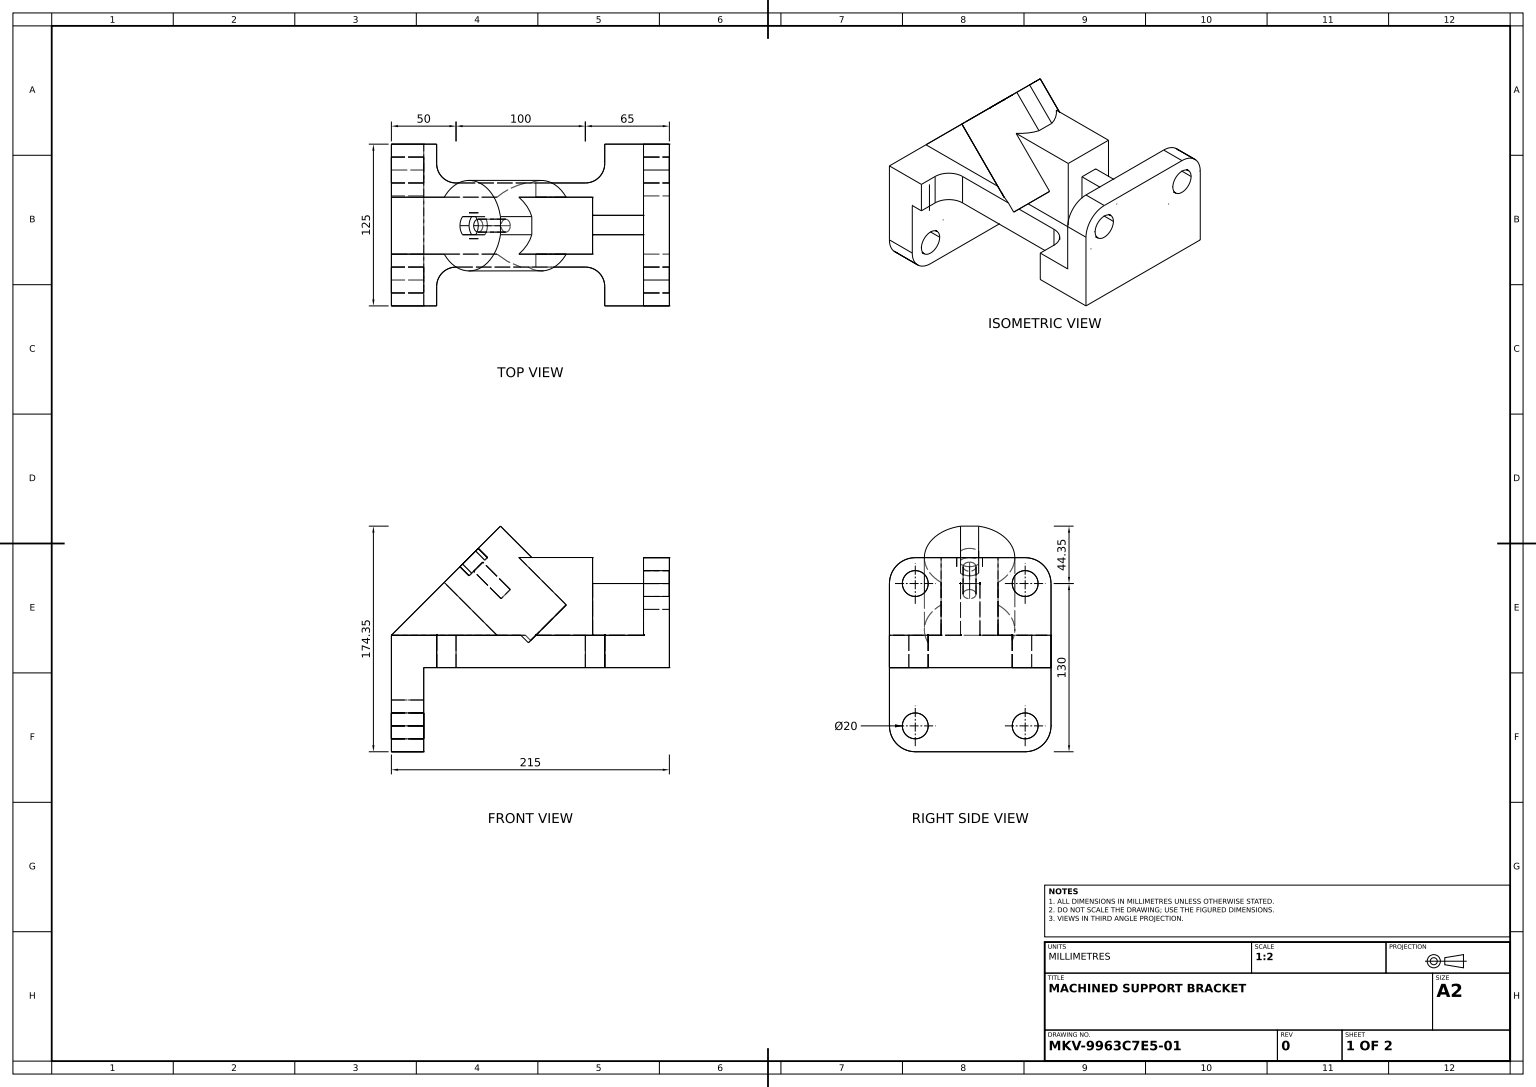
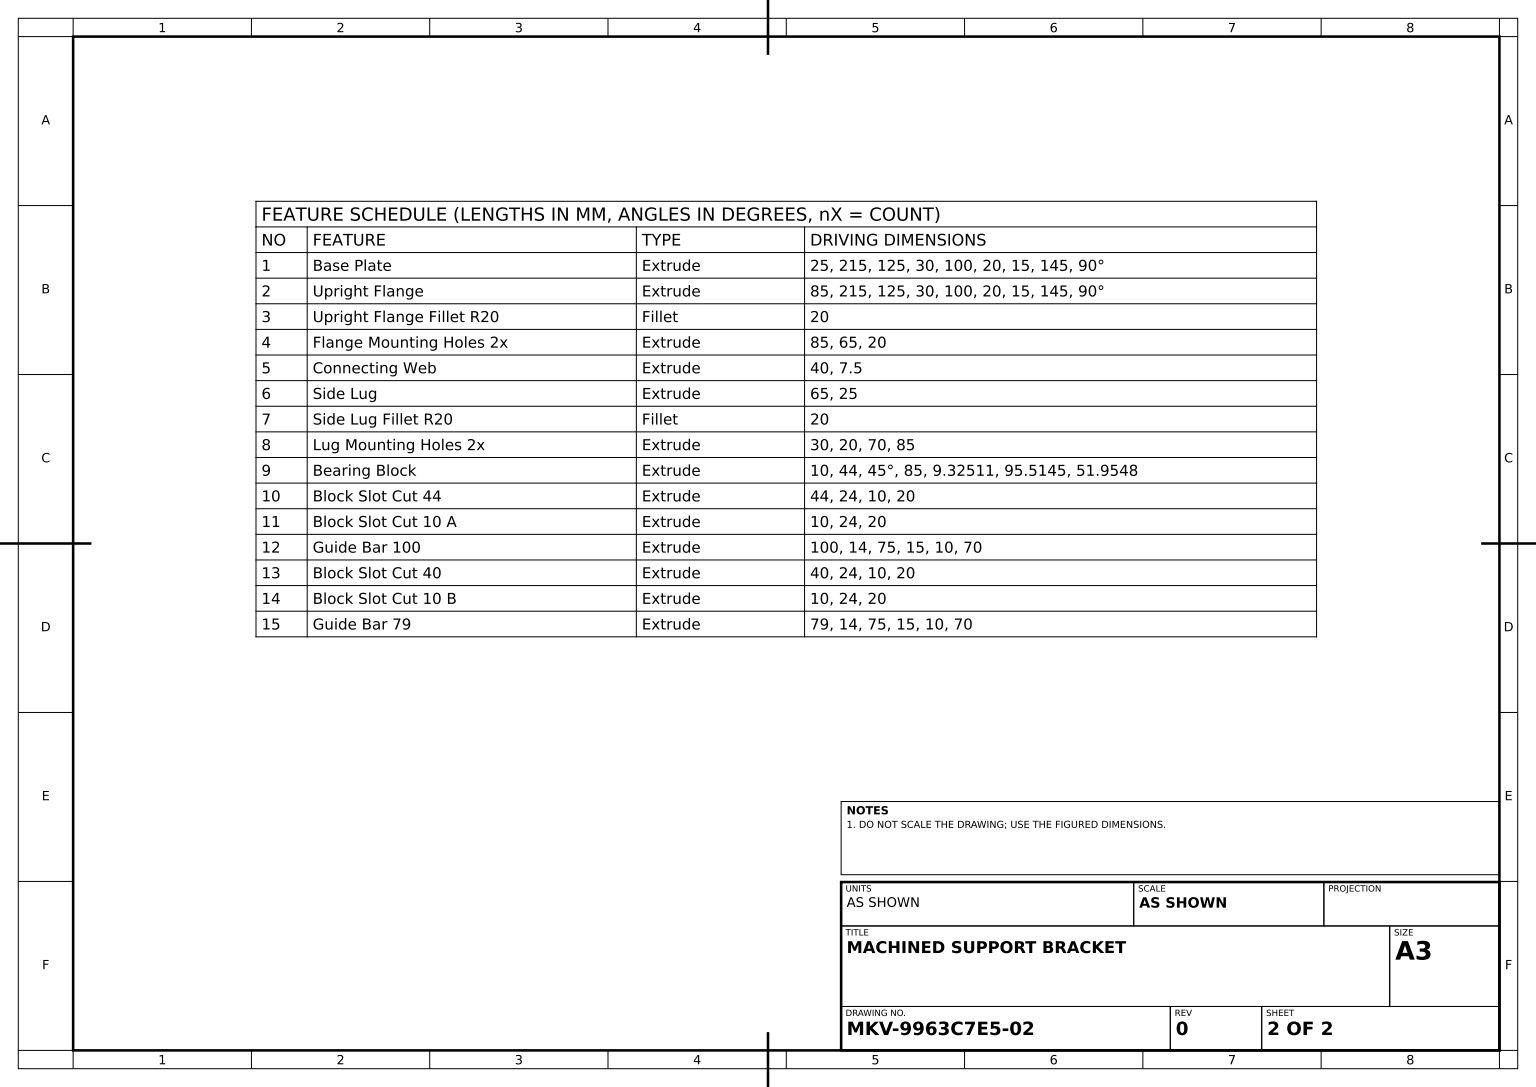
from build123d import *
from build123d.topology import SkipClean

# Parameters (mm, degrees)
BASE_PLATE_DEPTH               = 25
SKETCH1_3_W                    = 20
SKETCH1_3_H                    = 62.5
UPRIGHT_FLANGE_DEPTH           = 85
UPRIGHT_FLANGE_FILLET_R20_R    = 20
FLANGE_HOLES_SKETCH_R          = 10
FLANGE_MOUNTING_HOLES_2X_DEPTH = 85
CONNECTING_WEB_SKETCH_W        = 40
CONNECTING_WEB_SKETCH_H        = 15
CONNECTING_WEB_DEPTH           = 40
SIDE_LUG_SKETCH_W              = 25
SIDE_LUG_SKETCH_H              = 125
SIDE_LUG_DEPTH                 = 65
SIDE_LUG_FILLET_R20_R          = 20
LUG_HOLES_SKETCH_R             = 10
LUG_MOUNTING_HOLES_2X_DEPTH    = 30
BEARING_BLOCK_DEPTH            = 44
BLOCK_SLOT_SKETCH_R            = 5
BLOCK_SLOT_CUT_44_DEPTH        = 44
SKETCH12_4_R                   = 10
SKETCH12_4_R_2                 = 5
BLOCK_SLOT_CUT_10_A_DEPTH      = 10
GUIDE_BAR_SKETCH_W             = 14
GUIDE_BAR_SKETCH_H             = 44.292856399
GUIDE_BAR_100_DEPTH            = 100
SKETCH12_5_R                   = 5
BLOCK_SLOT_CUT_40_DEPTH        = 40
SKETCH12_6_R                   = 10
SKETCH12_6_R_2                 = 5
BLOCK_SLOT_CUT_10_B_DEPTH      = 10
GUIDE_BAR_79_DEPTH             = 79


with BuildPart() as part:
    # Base Profile Sketch → Base Plate (new body)
    with BuildSketch(Plane(origin=(0, 0, 0), x_dir=(1, 0, 0), z_dir=(0, 1, 0))):
        with BuildLine():
            Line((0, 62.5), (0, 0))
            Line((0, 0), (35, 0))
            Line((35, 0), (35, 15))
            ThreePointArc((35, 15), (39.393398282, 25.606601718), (50, 30))
            Line((50, 30), (150, 30))
            ThreePointArc((150, 30), (160.606601718, 25.606601718), (165, 15))
            Line((165, 15), (165, 0))
            Line((165, 0), (195, 0))
            Line((195, 0), (195, 62.5))
            Line((195, 62.5), (0, 62.5))
        make_face()
        with BuildLine():
            Line((0, 125), (0, 62.5))
            Line((0, 62.5), (195, 62.5))
            Line((195, 62.5), (195, 125))
            Line((195, 125), (165, 125))
            Line((165, 125), (165, 110))
            ThreePointArc((165, 110), (160.606601718, 99.393398282), (150, 95))
            Line((150, 95), (50, 95))
            ThreePointArc((50, 95), (39.393398282, 99.393398282), (35, 110))
            Line((35, 110), (35, 125))
            Line((35, 125), (0, 125))
        make_face()
    extrude(amount=BASE_PLATE_DEPTH)

    # Sketch1_3 → Upright Flange (add)
    with BuildSketch(Plane(origin=(0, 0, 0), x_dir=(1, 0, 0), z_dir=(0, 1, 0))):
        with Locations((205, 31.25)):
            Rectangle(SKETCH1_3_W, SKETCH1_3_H)
        with Locations((205, 93.75)):
            Rectangle(SKETCH1_3_W, SKETCH1_3_H)
    extrude(amount=UPRIGHT_FLANGE_DEPTH)

    # Upright Flange Fillet R20
    upright_flange_fillet_r20_edges = [part.edges().sort_by_distance(p)[0] for p in [
        (205, 85, 0),
        (205, 85, -125),
    ]]
    fillet(upright_flange_fillet_r20_edges, radius=UPRIGHT_FLANGE_FILLET_R20_R)

    # Flange Holes Sketch → Flange Mounting Holes 2x (cut)
    with BuildSketch(Plane(origin=(215, 0, 0), x_dir=(0, 0, -1), z_dir=(1, 0, 0))):
        with Locations((20, 65)):
            Circle(FLANGE_HOLES_SKETCH_R)
        with Locations((105, 65)):
            Circle(FLANGE_HOLES_SKETCH_R)
    extrude(amount=-FLANGE_MOUNTING_HOLES_2X_DEPTH, mode=Mode.SUBTRACT)

    # Connecting Web Sketch → Connecting Web (add)
    with BuildSketch(Plane(origin=(0, 25, 0), x_dir=(1, 0, 0), z_dir=(0, 1, 0))):
        with Locations((175, 62.5)):
            Rectangle(CONNECTING_WEB_SKETCH_W, CONNECTING_WEB_SKETCH_H)
    extrude(amount=CONNECTING_WEB_DEPTH)

    # Side Lug Sketch → Side Lug (add)
    with BuildSketch(Plane(origin=(0, 0, 0), x_dir=(-1, 0, 0), z_dir=(0, -1, 0))):
        with Locations((-12.5, 62.5)):
            Rectangle(SIDE_LUG_SKETCH_W, SIDE_LUG_SKETCH_H)
    extrude(amount=SIDE_LUG_DEPTH)

    # Side Lug Fillet R20
    side_lug_fillet_r20_edges = [part.edges().sort_by_distance(p)[0] for p in [
        (12.5, -65, 0),
        (12.5, -65, -125),
    ]]
    fillet(side_lug_fillet_r20_edges, radius=SIDE_LUG_FILLET_R20_R)

    # Lug Holes Sketch → Lug Mounting Holes 2x (cut)
    with BuildSketch(Plane.ZY):
        with Locations((-105, -45)):
            Circle(LUG_HOLES_SKETCH_R)
        with Locations((-20, -45)):
            Circle(LUG_HOLES_SKETCH_R)
    extrude(amount=-LUG_MOUNTING_HOLES_2X_DEPTH, mode=Mode.SUBTRACT)

    # Bearing Block Profile Sketch → Bearing Block (add)
    with BuildSketch(Plane.XY.offset(-40)):
        Polygon((0, 25), (60.104076401, 85.104076401), (146.293439814, 85.104076401), (155.618552468, 85.104076401), (155.618552468, 76.954753414), (155.618552468, 25), align=None)
    extrude(amount=-BEARING_BLOCK_DEPTH)

    # Block Slot Sketch → Block Slot Cut 44 (cut)
    with BuildSketch(Plane(origin=(-12.5, 12.5, 0), x_dir=(0, 0, 1), z_dir=(-0.7071067811865488, 0.7071067811865464, 0))):
        with Locations(Location((-62, 102.67766953, 0), (0, 0, 270))):
            Circle(BLOCK_SLOT_SKETCH_R)
    extrude(amount=-BLOCK_SLOT_CUT_44_DEPTH, mode=Mode.SUBTRACT)

    # Sketch12_4 → Block Slot Cut 10 A (cut)
    with SkipClean():  # the faces are left unmerged after this step: merging them gives an invalid solid
        with BuildSketch(Plane(origin=(-12.5, 12.5, 0), x_dir=(0, 0, 1), z_dir=(-0.7071067811865488, 0.7071067811865464, 0))):
            with Locations((-62, 102.67766953)):
                Circle(SKETCH12_4_R)
            with Locations((-62, 102.67766953)):
                Circle(SKETCH12_4_R_2, mode=Mode.SUBTRACT)
        extrude(amount=-BLOCK_SLOT_CUT_10_A_DEPTH, mode=Mode.SUBTRACT)

    # Guide Bar Sketch → Guide Bar 100 (add)
    with BuildSketch(Plane(origin=(-12.5, 12.5, 0), x_dir=(0, 0, 1), z_dir=(-0.7071067811865488, 0.7071067811865464, 0))):
        with Locations((-62, 114.82409773)):
            Rectangle(GUIDE_BAR_SKETCH_W, GUIDE_BAR_SKETCH_H)
    extrude(amount=-GUIDE_BAR_100_DEPTH)

    # Sketch12_5 → Block Slot Cut 40 (cut)
    with BuildSketch(Plane(origin=(-12.5, 12.5, 0), x_dir=(0, 0, 1), z_dir=(-0.7071067811865488, 0.7071067811865464, 0))):
        with Locations(Location((-62, 102.67766953, 0), (0, 0, 270))):
            Circle(SKETCH12_5_R)
    extrude(amount=-BLOCK_SLOT_CUT_40_DEPTH, mode=Mode.SUBTRACT)

    # Sketch12_6 → Block Slot Cut 10 B (cut)
    with BuildSketch(Plane(origin=(-12.5, 12.5, 0), x_dir=(0, 0, 1), z_dir=(-0.7071067811865488, 0.7071067811865464, 0))):
        with Locations(Location((-62, 102.67766953, 0), (0, 0, 270))):
            Circle(SKETCH12_6_R)
        with Locations(Location((-62, 102.67766953, 0), (0, 0, 270))):
            Circle(SKETCH12_6_R_2, mode=Mode.SUBTRACT)
    extrude(amount=-BLOCK_SLOT_CUT_10_B_DEPTH, mode=Mode.SUBTRACT)

    # Sketch13_6 → Guide Bar 79 (add)
    with BuildSketch(Plane(origin=(-12.5, 12.5, 0), x_dir=(0, 0, 1), z_dir=(-0.7071067811865488, 0.7071067811865464, 0))):
        with BuildLine():
            Line((-55, 136.970525929), (-55, 95.536241101))
            ThreePointArc((-55, 95.536241101), (-52.780455543, 98.804686183), (-52, 102.67766953))
            Line((-52, 102.67766953), (-40, 102.67766953))
            Line((-40, 102.67766953), (-40, 75.456354352))
            ThreePointArc((-40, 75.456354352), (-30.416776605, 87.594566401), (-27, 102.67766953))
            ThreePointArc((-27, 102.67766953), (-34.889116577, 124.813613151), (-55, 136.970525929))
        make_face()
        with BuildLine():
            ThreePointArc((-72, 102.67766953), (-71.219544457, 98.804686183), (-69, 95.536241101))
            Line((-69, 95.536241101), (-69, 136.970525929))
            ThreePointArc((-69, 136.970525929), (-96.00365166, 110.96933244), (-84, 75.456354352))
            Line((-84, 75.456354352), (-84, 102.67766953))
            Line((-84, 102.67766953), (-72, 102.67766953))
        make_face()
    extrude(amount=-GUIDE_BAR_79_DEPTH)


solid = part.part
